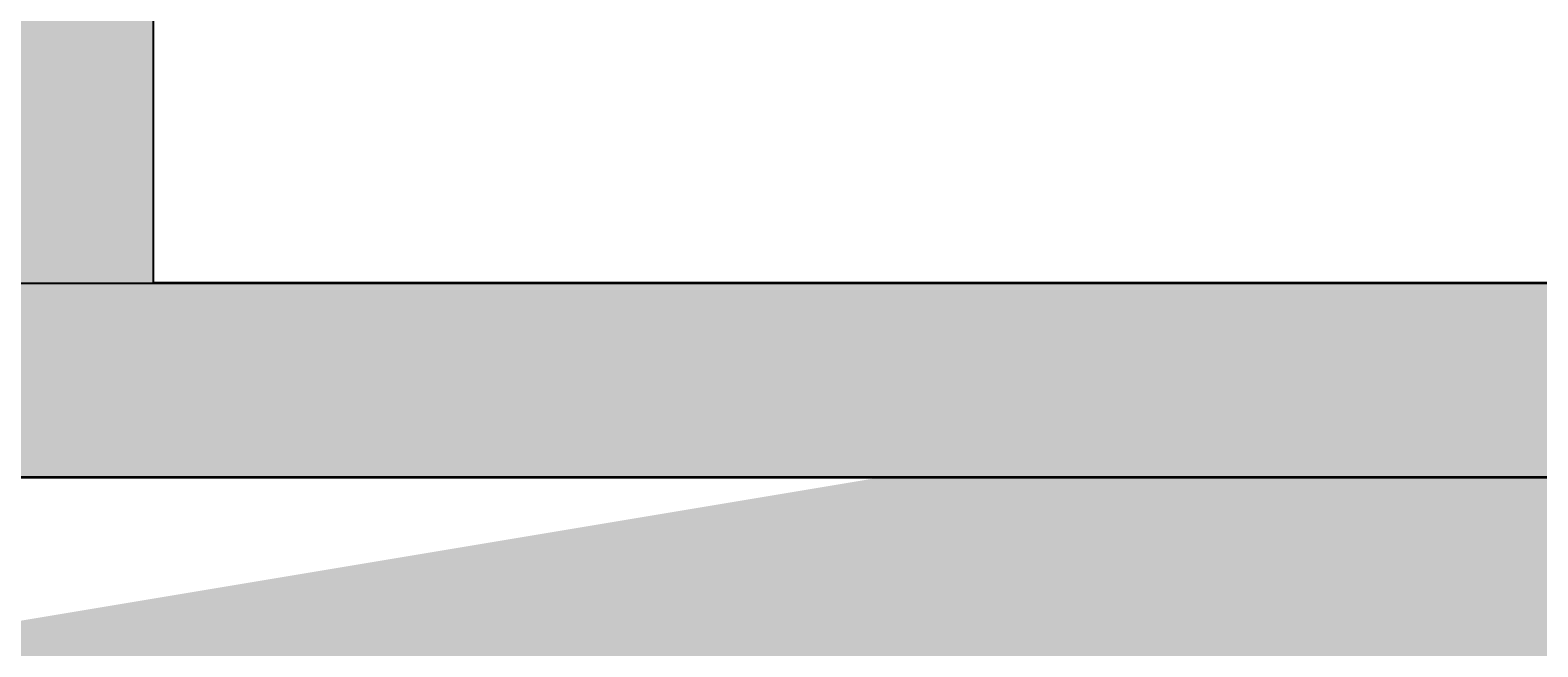
# Model space of a CAD drawing. Units: millimetres. Extents: x -22994 to 29398, y -19990 to 20176.
# Tile 51 of 135: x 198 to 247, y 5 to 25. Entities that reach past the tile are written whole.
import ezdxf

# ---------------------------------------------------------------- set-up
doc = ezdxf.new("R2010")
doc.units = ezdxf.units.MM
doc.header["$MEASUREMENT"] = 0
for name, color, linetype, lineweight in [('M-DIMS', 2, 'Continuous', 18), ('M-EQPM', 7, 'Continuous', 25), ('M-EQPM-PATT', 7, 'Continuous', 18), ('S-FNDN', 7, 'Continuous', 35)]:
    doc.layers.add(name, color=color, linetype=linetype, lineweight=lineweight)
doc.styles.get("Standard").update_dxf_attribs({"font": 'arial.ttf'})
doc.dimstyles.get("Standard").update_dxf_attribs({"dimtxt": 0.18, "dimasz": 10000, "dimexe": 0.18, "dimexo": 0.0625, "dimgap": 0.09, "dimtad": 0, "dimtih": 1, "dimtoh": 1, "dimdec": 0, "dimzin": 0, "dimdsep": 46, "dimtxsty": 'Standard', "dimcen": 0.09, "dimadec": 0, "dimazin": 0, "dimtfac": 1, "dimtdec": 0, "dimtofl": 0, "dimtmove": 0, "dimatfit": 3, "dimfxl": 1, "dimtolj": 1, "dimtzin": 0, "dimlwd": 30, "dimarcsym": 0})

# ---------------------------------------------------------------- blocks, each defined once
blk = doc.blocks.new('*D2')
at = {"layer": 'Defpoints', "color": 0, "transparency": 16777216}
for p in [(6.677, 10.271), (290.852, 10.271), (290.852, -5.079)]:
    blk.add_point(p, dxfattribs=at)
at = {"layer": 'M-DIMS', "color": 0, "lineweight": -2, "transparency": 16777216}
for p, q in [((6.677, 10.209), (6.677, -5.259)), ((290.852, 10.209), (290.852, -5.259))]:
    blk.add_line(p, q, dxfattribs=at)
at = {"layer": 'M-DIMS', "color": 0, "lineweight": 30, "transparency": 16777216}
for p, q in [((-9993.323, -5.079), (-19993.323, -5.079)), ((10290.852, -5.079), (20290.852, -5.079))]:
    blk.add_line(p, q, dxfattribs=at)
at = {"layer": 'M-DIMS', "color": 0, "transparency": 16777216}
for points in [[(-9993.323, 1661.588), (-9993.323, -1671.745), (6.677, -5.079)], [(10290.852, 1661.588), (10290.852, -1671.745), (290.852, -5.079)]]:
    blk.add_solid(points, dxfattribs=at)
at = {"layer": 'M-DIMS', "color": 0, "transparency": 16777216, "insert": (148.765, -5.079), "char_height": 0.18, "attachment_point": 5}
blk.add_mtext('\\A1;284.2', dxfattribs=at)
blk = doc.blocks.new('*D3')
at = {"layer": 'Defpoints', "color": 0, "transparency": 16777216}
for p in [(110.265, 204.165), (110.265, 176.366), (95.833, 127.967)]:
    blk.add_point(p, dxfattribs=at)
at = {"layer": 'M-DIMS', "color": 0, "lineweight": -2, "transparency": 16777216}
for p, q in [((95.833, 128.03), (95.833, 204.345)), ((110.265, 176.429), (110.265, 204.345))]:
    blk.add_line(p, q, dxfattribs=at)
at = {"layer": 'M-DIMS', "color": 0, "lineweight": 30, "transparency": 16777216}
for p, q in [((-9904.167, 204.165), (-19904.167, 204.165)), ((10110.265, 204.165), (20110.265, 204.165))]:
    blk.add_line(p, q, dxfattribs=at)
at = {"layer": 'M-DIMS', "color": 0, "transparency": 16777216}
for points in [[(-9904.167, 1870.832), (-9904.167, -1462.501), (95.833, 204.165)], [(10110.265, 1870.832), (10110.265, -1462.501), (110.265, 204.165)]]:
    blk.add_solid(points, dxfattribs=at)
at = {"layer": 'M-DIMS', "color": 0, "transparency": 16777216, "insert": (103.049, 204.165), "char_height": 0.18, "attachment_point": 5}
blk.add_mtext('\\A1;14.432', dxfattribs=at)
blk = doc.blocks.new('*D4')
at = {"layer": 'Defpoints', "color": 0, "transparency": 16777216}
for p in [(116.265, 204.165), (110.265, 176.366), (116.265, 176.366)]:
    blk.add_point(p, dxfattribs=at)
at = {"layer": 'M-DIMS', "color": 0, "lineweight": -2, "transparency": 16777216}
for p, q in [((110.265, 176.429), (110.265, 204.345)), ((116.265, 176.429), (116.265, 204.345))]:
    blk.add_line(p, q, dxfattribs=at)
at = {"layer": 'M-DIMS', "color": 0, "lineweight": 30, "transparency": 16777216}
for p, q in [((-9889.735, 204.165), (-19889.735, 204.165)), ((10116.265, 204.165), (20116.265, 204.165))]:
    blk.add_line(p, q, dxfattribs=at)
at = {"layer": 'M-DIMS', "color": 0, "transparency": 16777216}
for points in [[(-9889.735, 1870.832), (-9889.735, -1462.501), (110.265, 204.165)], [(10116.265, 1870.832), (10116.265, -1462.501), (116.265, 204.165)]]:
    blk.add_solid(points, dxfattribs=at)
at = {"layer": 'M-DIMS', "color": 0, "transparency": 16777216, "insert": (113.265, 204.165), "char_height": 0.18, "attachment_point": 5}
blk.add_mtext('\\A1;6', dxfattribs=at)
blk = doc.blocks.new('*D5')
at = {"layer": 'Defpoints', "color": 0, "transparency": 16777216}
for p in [(181.265, 204.165), (116.265, 176.366), (181.265, 176.366)]:
    blk.add_point(p, dxfattribs=at)
at = {"layer": 'M-DIMS', "color": 0, "lineweight": -2, "transparency": 16777216}
for p, q in [((116.265, 176.429), (116.265, 204.345)), ((181.265, 176.429), (181.265, 204.345))]:
    blk.add_line(p, q, dxfattribs=at)
at = {"layer": 'M-DIMS', "color": 0, "lineweight": 30, "transparency": 16777216}
for p, q in [((-9883.735, 204.165), (-19883.735, 204.165)), ((10181.265, 204.165), (20181.265, 204.165))]:
    blk.add_line(p, q, dxfattribs=at)
at = {"layer": 'M-DIMS', "color": 0, "transparency": 16777216}
for points in [[(-9883.735, 1870.832), (-9883.735, -1462.501), (116.265, 204.165)], [(10181.265, 1870.832), (10181.265, -1462.501), (181.265, 204.165)]]:
    blk.add_solid(points, dxfattribs=at)
at = {"layer": 'M-DIMS', "color": 0, "transparency": 16777216, "insert": (148.765, 204.165), "char_height": 0.18, "attachment_point": 5}
blk.add_mtext('\\A1;65', dxfattribs=at)
blk = doc.blocks.new('*D6')
at = {"layer": 'Defpoints', "color": 0, "transparency": 16777216}
for p in [(187.265, 204.165), (181.265, 176.366), (187.265, 176.366)]:
    blk.add_point(p, dxfattribs=at)
at = {"layer": 'M-DIMS', "color": 0, "lineweight": -2, "transparency": 16777216}
for p, q in [((181.265, 176.429), (181.265, 204.345)), ((187.265, 176.429), (187.265, 204.345))]:
    blk.add_line(p, q, dxfattribs=at)
at = {"layer": 'M-DIMS', "color": 0, "lineweight": 30, "transparency": 16777216}
for p, q in [((-9818.735, 204.165), (-19818.735, 204.165)), ((10187.265, 204.165), (20187.265, 204.165))]:
    blk.add_line(p, q, dxfattribs=at)
at = {"layer": 'M-DIMS', "color": 0, "transparency": 16777216}
for points in [[(-9818.735, 1870.832), (-9818.735, -1462.501), (181.265, 204.165)], [(10187.265, 1870.832), (10187.265, -1462.501), (187.265, 204.165)]]:
    blk.add_solid(points, dxfattribs=at)
at = {"layer": 'M-DIMS', "color": 0, "transparency": 16777216, "insert": (184.265, 204.165), "char_height": 0.18, "attachment_point": 5}
blk.add_mtext('\\A1;6', dxfattribs=at)
blk = doc.blocks.new('*D7')
at = {"layer": 'Defpoints', "color": 0, "transparency": 16777216}
for p in [(201.697, 204.165), (187.265, 176.366), (201.697, 127.967)]:
    blk.add_point(p, dxfattribs=at)
at = {"layer": 'M-DIMS', "color": 0, "lineweight": -2, "transparency": 16777216}
for p, q in [((187.265, 176.429), (187.265, 204.345)), ((201.697, 128.03), (201.697, 204.345))]:
    blk.add_line(p, q, dxfattribs=at)
at = {"layer": 'M-DIMS', "color": 0, "lineweight": 30, "transparency": 16777216}
for p, q in [((-9812.735, 204.165), (-19812.735, 204.165)), ((10201.697, 204.165), (20201.697, 204.165))]:
    blk.add_line(p, q, dxfattribs=at)
at = {"layer": 'M-DIMS', "color": 0, "transparency": 16777216}
for points in [[(-9812.735, 1870.832), (-9812.735, -1462.501), (187.265, 204.165)], [(10201.697, 1870.832), (10201.697, -1462.501), (201.697, 204.165)]]:
    blk.add_solid(points, dxfattribs=at)
at = {"layer": 'M-DIMS', "color": 0, "transparency": 16777216, "insert": (194.481, 204.165), "char_height": 0.18, "attachment_point": 5}
blk.add_mtext('\\A1;14.432', dxfattribs=at)
blk = doc.blocks.new('*D8')
at = {"layer": 'Defpoints', "color": 0, "transparency": 16777216}
for p in [(227.648, 204.165), (227.648, 146.73), (201.697, 127.967)]:
    blk.add_point(p, dxfattribs=at)
at = {"layer": 'M-DIMS', "color": 0, "lineweight": -2, "transparency": 16777216}
for p, q in [((201.697, 128.03), (201.697, 204.345)), ((227.648, 146.792), (227.648, 204.345))]:
    blk.add_line(p, q, dxfattribs=at)
at = {"layer": 'M-DIMS', "color": 0, "lineweight": 30, "transparency": 16777216}
for p, q in [((-9798.303, 204.165), (-19798.303, 204.165)), ((10227.648, 204.165), (20227.648, 204.165))]:
    blk.add_line(p, q, dxfattribs=at)
at = {"layer": 'M-DIMS', "color": 0, "transparency": 16777216}
for points in [[(-9798.303, 1870.832), (-9798.303, -1462.501), (201.697, 204.165)], [(10227.648, 1870.832), (10227.648, -1462.501), (227.648, 204.165)]]:
    blk.add_solid(points, dxfattribs=at)
at = {"layer": 'M-DIMS', "color": 0, "transparency": 16777216, "insert": (214.673, 204.165), "char_height": 0.18, "attachment_point": 5}
blk.add_mtext('\\A1;25.95', dxfattribs=at)
blk = doc.blocks.new('*D9')
at = {"layer": 'Defpoints', "color": 0, "transparency": 16777216}
for p in [(187.265, 176.366), (306.202, 176.366), (290.852, 10.271)]:
    blk.add_point(p, dxfattribs=at)
at = {"layer": 'M-DIMS', "color": 0, "lineweight": 30, "transparency": 16777216}
for p, q in [((306.202, 10176.366), (306.202, 20176.366)), ((306.202, -9989.729), (306.202, -19989.729))]:
    blk.add_line(p, q, dxfattribs=at)
at = {"layer": 'M-DIMS', "color": 0, "lineweight": -2, "transparency": 16777216}
for p, q in [((187.327, 176.366), (306.382, 176.366)), ((290.915, 10.271), (306.382, 10.271))]:
    blk.add_line(p, q, dxfattribs=at)
at = {"layer": 'M-DIMS', "color": 0, "transparency": 16777216}
for points in [[(-1360.465, 10176.366), (1972.869, 10176.366), (306.202, 176.366)], [(-1360.465, -9989.729), (1972.869, -9989.729), (306.202, 10.271)]]:
    blk.add_solid(points, dxfattribs=at)
at = {"layer": 'M-DIMS', "color": 0, "transparency": 16777216, "insert": (306.202, 93.319), "char_height": 0.18, "attachment_point": 5}
blk.add_mtext('\\A1;166.1', dxfattribs=at)
blk = doc.blocks.new('*D10')
at = {"layer": 'Defpoints', "color": 0, "transparency": 16777216}
for p in [(125.65, 136.071), (133.346, 136.071), (133.346, -5.079)]:
    blk.add_point(p, dxfattribs=at)
at = {"layer": 'M-DIMS', "color": 0, "lineweight": -2, "transparency": 16777216}
for p, q in [((125.65, 136.009), (125.65, -5.259)), ((133.346, 136.009), (133.346, -5.259))]:
    blk.add_line(p, q, dxfattribs=at)
at = {"layer": 'M-DIMS', "color": 0, "lineweight": 30, "transparency": 16777216}
for p, q in [((-9874.35, -5.079), (-19874.35, -5.079)), ((10133.346, -5.079), (20133.346, -5.079))]:
    blk.add_line(p, q, dxfattribs=at)
at = {"layer": 'M-DIMS', "color": 0, "transparency": 16777216}
for points in [[(-9874.35, 1661.588), (-9874.35, -1671.745), (125.65, -5.079)], [(10133.346, 1661.588), (10133.346, -1671.745), (133.346, -5.079)]]:
    blk.add_solid(points, dxfattribs=at)
at = {"layer": 'M-DIMS', "color": 0, "transparency": 16777216, "insert": (129.498, -5.079), "char_height": 0.18, "attachment_point": 5}
blk.add_mtext('\\A1;7.696', dxfattribs=at)
blk = doc.blocks.new('*D11')
at = {"layer": 'Defpoints', "color": 0, "transparency": 16777216}
for p in [(133.346, 136.071), (135.65, 136.071), (135.65, -5.079)]:
    blk.add_point(p, dxfattribs=at)
at = {"layer": 'M-DIMS', "color": 0, "lineweight": -2, "transparency": 16777216}
for p, q in [((133.346, 136.009), (133.346, -5.259)), ((135.65, 136.009), (135.65, -5.259))]:
    blk.add_line(p, q, dxfattribs=at)
at = {"layer": 'M-DIMS', "color": 0, "lineweight": 30, "transparency": 16777216}
for p, q in [((-9866.654, -5.079), (-19866.654, -5.079)), ((10135.65, -5.079), (20135.65, -5.079))]:
    blk.add_line(p, q, dxfattribs=at)
at = {"layer": 'M-DIMS', "color": 0, "transparency": 16777216}
for points in [[(-9866.654, 1661.588), (-9866.654, -1671.745), (133.346, -5.079)], [(10135.65, 1661.588), (10135.65, -1671.745), (135.65, -5.079)]]:
    blk.add_solid(points, dxfattribs=at)
at = {"layer": 'M-DIMS', "color": 0, "transparency": 16777216, "insert": (134.498, -5.079), "char_height": 0.18, "attachment_point": 5}
blk.add_mtext('\\A1;2.304', dxfattribs=at)
blk = doc.blocks.new('*D12')
at = {"layer": 'Defpoints', "color": 0, "transparency": 16777216}
for p in [(135.65, 136.071), (145.65, 136.071), (145.65, -5.079)]:
    blk.add_point(p, dxfattribs=at)
at = {"layer": 'M-DIMS', "color": 0, "lineweight": -2, "transparency": 16777216}
for p, q in [((135.65, 136.009), (135.65, -5.259)), ((145.65, 136.009), (145.65, -5.259))]:
    blk.add_line(p, q, dxfattribs=at)
at = {"layer": 'M-DIMS', "color": 0, "lineweight": 30, "transparency": 16777216}
for p, q in [((-9864.35, -5.079), (-19864.35, -5.079)), ((10145.65, -5.079), (20145.65, -5.079))]:
    blk.add_line(p, q, dxfattribs=at)
at = {"layer": 'M-DIMS', "color": 0, "transparency": 16777216}
for points in [[(-9864.35, 1661.588), (-9864.35, -1671.745), (135.65, -5.079)], [(10145.65, 1661.588), (10145.65, -1671.745), (145.65, -5.079)]]:
    blk.add_solid(points, dxfattribs=at)
at = {"layer": 'M-DIMS', "color": 0, "transparency": 16777216, "insert": (140.65, -5.079), "char_height": 0.18, "attachment_point": 5}
blk.add_mtext('\\A1;10', dxfattribs=at)
blk = doc.blocks.new('*D13')
at = {"layer": 'Defpoints', "color": 0, "transparency": 16777216}
for p in [(145.65, 136.071), (155.65, 136.071), (155.65, -5.079)]:
    blk.add_point(p, dxfattribs=at)
at = {"layer": 'M-DIMS', "color": 0, "lineweight": -2, "transparency": 16777216}
for p, q in [((145.65, 136.009), (145.65, -5.259)), ((155.65, 136.009), (155.65, -5.259))]:
    blk.add_line(p, q, dxfattribs=at)
at = {"layer": 'M-DIMS', "color": 0, "lineweight": 30, "transparency": 16777216}
for p, q in [((-9854.35, -5.079), (-19854.35, -5.079)), ((10155.65, -5.079), (20155.65, -5.079))]:
    blk.add_line(p, q, dxfattribs=at)
at = {"layer": 'M-DIMS', "color": 0, "transparency": 16777216}
for points in [[(-9854.35, 1661.588), (-9854.35, -1671.745), (145.65, -5.079)], [(10155.65, 1661.588), (10155.65, -1671.745), (155.65, -5.079)]]:
    blk.add_solid(points, dxfattribs=at)
at = {"layer": 'M-DIMS', "color": 0, "transparency": 16777216, "insert": (150.65, -5.079), "char_height": 0.18, "attachment_point": 5}
blk.add_mtext('\\A1;10', dxfattribs=at)
blk = doc.blocks.new('*D14')
at = {"layer": 'Defpoints', "color": 0, "transparency": 16777216}
for p in [(155.65, 136.071), (165.65, 136.071), (165.65, -5.079)]:
    blk.add_point(p, dxfattribs=at)
at = {"layer": 'M-DIMS', "color": 0, "lineweight": -2, "transparency": 16777216}
for p, q in [((155.65, 136.009), (155.65, -5.259)), ((165.65, 136.009), (165.65, -5.259))]:
    blk.add_line(p, q, dxfattribs=at)
at = {"layer": 'M-DIMS', "color": 0, "lineweight": 30, "transparency": 16777216}
for p, q in [((-9844.35, -5.079), (-19844.35, -5.079)), ((10165.65, -5.079), (20165.65, -5.079))]:
    blk.add_line(p, q, dxfattribs=at)
at = {"layer": 'M-DIMS', "color": 0, "transparency": 16777216}
for points in [[(-9844.35, 1661.588), (-9844.35, -1671.745), (155.65, -5.079)], [(10165.65, 1661.588), (10165.65, -1671.745), (165.65, -5.079)]]:
    blk.add_solid(points, dxfattribs=at)
at = {"layer": 'M-DIMS', "color": 0, "transparency": 16777216, "insert": (160.65, -5.079), "char_height": 0.18, "attachment_point": 5}
blk.add_mtext('\\A1;10', dxfattribs=at)
blk = doc.blocks.new('*D15')
at = {"layer": 'Defpoints', "color": 0, "transparency": 16777216}
for p in [(173.346, 154.788), (173.346, 136.071), (306.202, 136.071)]:
    blk.add_point(p, dxfattribs=at)
at = {"layer": 'M-DIMS', "color": 0, "lineweight": 30, "transparency": 16777216}
for p, q in [((306.202, 10154.788), (306.202, 20154.788)), ((306.202, -9863.929), (306.202, -19863.929))]:
    blk.add_line(p, q, dxfattribs=at)
at = {"layer": 'M-DIMS', "color": 0, "lineweight": -2, "transparency": 16777216}
for p, q in [((173.408, 154.788), (306.382, 154.788)), ((173.408, 136.071), (306.382, 136.071))]:
    blk.add_line(p, q, dxfattribs=at)
at = {"layer": 'M-DIMS', "color": 0, "transparency": 16777216}
for points in [[(-1360.465, 10154.788), (1972.869, 10154.788), (306.202, 154.788)], [(-1360.465, -9863.929), (1972.869, -9863.929), (306.202, 136.071)]]:
    blk.add_solid(points, dxfattribs=at)
at = {"layer": 'M-DIMS', "color": 0, "transparency": 16777216, "insert": (306.202, 145.43), "char_height": 0.18, "attachment_point": 5}
blk.add_mtext('\\A1;18.717', dxfattribs=at)
blk = doc.blocks.new('*D16')
at = {"layer": 'Defpoints', "color": 0, "transparency": 16777216}
for p in [(120.17, 204.165), (110.466, 48.035), (120.17, 48.035)]:
    blk.add_point(p, dxfattribs=at)
at = {"layer": 'M-DIMS', "color": 0, "lineweight": -2, "transparency": 16777216}
for p, q in [((110.466, 48.097), (110.466, 204.345)), ((120.17, 48.097), (120.17, 204.345))]:
    blk.add_line(p, q, dxfattribs=at)
at = {"layer": 'M-DIMS', "color": 0, "lineweight": 30, "transparency": 16777216}
for p, q in [((-9889.534, 204.165), (-19889.534, 204.165)), ((10120.17, 204.165), (20120.17, 204.165))]:
    blk.add_line(p, q, dxfattribs=at)
at = {"layer": 'M-DIMS', "color": 0, "transparency": 16777216}
for points in [[(-9889.534, 1870.832), (-9889.534, -1462.501), (110.466, 204.165)], [(10120.17, 1870.832), (10120.17, -1462.501), (120.17, 204.165)]]:
    blk.add_solid(points, dxfattribs=at)
at = {"layer": 'M-DIMS', "color": 0, "transparency": 16777216, "insert": (115.318, 204.165), "char_height": 0.18, "attachment_point": 5}
blk.add_mtext('\\A1;9.704', dxfattribs=at)
blk = doc.blocks.new('*D17')
at = {"layer": 'Defpoints', "color": 0, "transparency": 16777216}
for p in [(126.17, 204.165), (120.17, 48.035), (126.17, 48.035)]:
    blk.add_point(p, dxfattribs=at)
at = {"layer": 'M-DIMS', "color": 0, "lineweight": -2, "transparency": 16777216}
for p, q in [((120.17, 48.097), (120.17, 204.345)), ((126.17, 48.097), (126.17, 204.345))]:
    blk.add_line(p, q, dxfattribs=at)
at = {"layer": 'M-DIMS', "color": 0, "lineweight": 30, "transparency": 16777216}
for p, q in [((-9879.83, 204.165), (-19879.83, 204.165)), ((10126.17, 204.165), (20126.17, 204.165))]:
    blk.add_line(p, q, dxfattribs=at)
at = {"layer": 'M-DIMS', "color": 0, "transparency": 16777216}
for points in [[(-9879.83, 1870.832), (-9879.83, -1462.501), (120.17, 204.165)], [(10126.17, 1870.832), (10126.17, -1462.501), (126.17, 204.165)]]:
    blk.add_solid(points, dxfattribs=at)
at = {"layer": 'M-DIMS', "color": 0, "transparency": 16777216, "insert": (123.17, 204.165), "char_height": 0.18, "attachment_point": 5}
blk.add_mtext('\\A1;6', dxfattribs=at)
blk = doc.blocks.new('*D18')
at = {"layer": 'Defpoints', "color": 0, "transparency": 16777216}
for p in [(132.17, 204.165), (126.17, 48.035), (132.17, 48.035)]:
    blk.add_point(p, dxfattribs=at)
at = {"layer": 'M-DIMS', "color": 0, "lineweight": -2, "transparency": 16777216}
for p, q in [((126.17, 48.097), (126.17, 204.345)), ((132.17, 48.097), (132.17, 204.345))]:
    blk.add_line(p, q, dxfattribs=at)
at = {"layer": 'M-DIMS', "color": 0, "lineweight": 30, "transparency": 16777216}
for p, q in [((-9873.83, 204.165), (-19873.83, 204.165)), ((10132.17, 204.165), (20132.17, 204.165))]:
    blk.add_line(p, q, dxfattribs=at)
at = {"layer": 'M-DIMS', "color": 0, "transparency": 16777216}
for points in [[(-9873.83, 1870.832), (-9873.83, -1462.501), (126.17, 204.165)], [(10132.17, 1870.832), (10132.17, -1462.501), (132.17, 204.165)]]:
    blk.add_solid(points, dxfattribs=at)
at = {"layer": 'M-DIMS', "color": 0, "transparency": 16777216, "insert": (129.17, 204.165), "char_height": 0.18, "attachment_point": 5}
blk.add_mtext('\\A1;6', dxfattribs=at)
blk = doc.blocks.new('*D19')
at = {"layer": 'Defpoints', "color": 0, "transparency": 16777216}
for p in [(138.17, 204.165), (132.17, 48.035), (138.17, 48.035)]:
    blk.add_point(p, dxfattribs=at)
at = {"layer": 'M-DIMS', "color": 0, "lineweight": -2, "transparency": 16777216}
for p, q in [((132.17, 48.097), (132.17, 204.345)), ((138.17, 48.097), (138.17, 204.345))]:
    blk.add_line(p, q, dxfattribs=at)
at = {"layer": 'M-DIMS', "color": 0, "lineweight": 30, "transparency": 16777216}
for p, q in [((-9867.83, 204.165), (-19867.83, 204.165)), ((10138.17, 204.165), (20138.17, 204.165))]:
    blk.add_line(p, q, dxfattribs=at)
at = {"layer": 'M-DIMS', "color": 0, "transparency": 16777216}
for points in [[(-9867.83, 1870.832), (-9867.83, -1462.501), (132.17, 204.165)], [(10138.17, 1870.832), (10138.17, -1462.501), (138.17, 204.165)]]:
    blk.add_solid(points, dxfattribs=at)
at = {"layer": 'M-DIMS', "color": 0, "transparency": 16777216, "insert": (135.17, 204.165), "char_height": 0.18, "attachment_point": 5}
blk.add_mtext('\\A1;6', dxfattribs=at)
blk = doc.blocks.new('*D20')
at = {"layer": 'Defpoints', "color": 0, "transparency": 16777216}
for p in [(144.17, 204.165), (138.17, 48.035), (144.17, 48.035)]:
    blk.add_point(p, dxfattribs=at)
at = {"layer": 'M-DIMS', "color": 0, "lineweight": -2, "transparency": 16777216}
for p, q in [((138.17, 48.097), (138.17, 204.345)), ((144.17, 48.097), (144.17, 204.345))]:
    blk.add_line(p, q, dxfattribs=at)
at = {"layer": 'M-DIMS', "color": 0, "lineweight": 30, "transparency": 16777216}
for p, q in [((-9861.83, 204.165), (-19861.83, 204.165)), ((10144.17, 204.165), (20144.17, 204.165))]:
    blk.add_line(p, q, dxfattribs=at)
at = {"layer": 'M-DIMS', "color": 0, "transparency": 16777216}
for points in [[(-9861.83, 1870.832), (-9861.83, -1462.501), (138.17, 204.165)], [(10144.17, 1870.832), (10144.17, -1462.501), (144.17, 204.165)]]:
    blk.add_solid(points, dxfattribs=at)
at = {"layer": 'M-DIMS', "color": 0, "transparency": 16777216, "insert": (141.17, 204.165), "char_height": 0.18, "attachment_point": 5}
blk.add_mtext('\\A1;6', dxfattribs=at)
blk = doc.blocks.new('*D21')
at = {"layer": 'Defpoints', "color": 0, "transparency": 16777216}
for p in [(149.116, 204.165), (144.17, 48.035), (149.116, 48.035)]:
    blk.add_point(p, dxfattribs=at)
at = {"layer": 'M-DIMS', "color": 0, "lineweight": -2, "transparency": 16777216}
for p, q in [((144.17, 48.097), (144.17, 204.345)), ((149.116, 48.097), (149.116, 204.345))]:
    blk.add_line(p, q, dxfattribs=at)
at = {"layer": 'M-DIMS', "color": 0, "lineweight": 30, "transparency": 16777216}
for p, q in [((-9855.83, 204.165), (-19855.83, 204.165)), ((10149.116, 204.165), (20149.116, 204.165))]:
    blk.add_line(p, q, dxfattribs=at)
at = {"layer": 'M-DIMS', "color": 0, "transparency": 16777216}
for points in [[(-9855.83, 1870.832), (-9855.83, -1462.501), (144.17, 204.165)], [(10149.116, 1870.832), (10149.116, -1462.501), (149.116, 204.165)]]:
    blk.add_solid(points, dxfattribs=at)
at = {"layer": 'M-DIMS', "color": 0, "transparency": 16777216, "insert": (146.643, 204.165), "char_height": 0.18, "attachment_point": 5}
blk.add_mtext('\\A1;4.945', dxfattribs=at)
blk = doc.blocks.new('*D22')
at = {"layer": 'Defpoints', "color": 0, "transparency": 16777216}
for p in [(149.116, 30.99), (155.116, 30.99), (155.116, -5.079)]:
    blk.add_point(p, dxfattribs=at)
at = {"layer": 'M-DIMS', "color": 0, "lineweight": -2, "transparency": 16777216}
for p, q in [((149.116, 30.927), (149.116, -5.259)), ((155.116, 30.927), (155.116, -5.259))]:
    blk.add_line(p, q, dxfattribs=at)
at = {"layer": 'M-DIMS', "color": 0, "lineweight": 30, "transparency": 16777216}
for p, q in [((-9850.884, -5.079), (-19850.884, -5.079)), ((10155.116, -5.079), (20155.116, -5.079))]:
    blk.add_line(p, q, dxfattribs=at)
at = {"layer": 'M-DIMS', "color": 0, "transparency": 16777216}
for points in [[(-9850.884, 1661.588), (-9850.884, -1671.745), (149.116, -5.079)], [(10155.116, 1661.588), (10155.116, -1671.745), (155.116, -5.079)]]:
    blk.add_solid(points, dxfattribs=at)
at = {"layer": 'M-DIMS', "color": 0, "transparency": 16777216, "insert": (152.116, -5.079), "char_height": 0.18, "attachment_point": 5}
blk.add_mtext('\\A1;6', dxfattribs=at)
blk = doc.blocks.new('*D23')
at = {"layer": 'Defpoints', "color": 0, "transparency": 16777216}
for p in [(155.116, 30.99), (161.116, 30.99), (161.116, -5.079)]:
    blk.add_point(p, dxfattribs=at)
at = {"layer": 'M-DIMS', "color": 0, "lineweight": -2, "transparency": 16777216}
for p, q in [((155.116, 30.927), (155.116, -5.259)), ((161.116, 30.927), (161.116, -5.259))]:
    blk.add_line(p, q, dxfattribs=at)
at = {"layer": 'M-DIMS', "color": 0, "lineweight": 30, "transparency": 16777216}
for p, q in [((-9844.884, -5.079), (-19844.884, -5.079)), ((10161.116, -5.079), (20161.116, -5.079))]:
    blk.add_line(p, q, dxfattribs=at)
at = {"layer": 'M-DIMS', "color": 0, "transparency": 16777216}
for points in [[(-9844.884, 1661.588), (-9844.884, -1671.745), (155.116, -5.079)], [(10161.116, 1661.588), (10161.116, -1671.745), (161.116, -5.079)]]:
    blk.add_solid(points, dxfattribs=at)
at = {"layer": 'M-DIMS', "color": 0, "transparency": 16777216, "insert": (158.116, -5.079), "char_height": 0.18, "attachment_point": 5}
blk.add_mtext('\\A1;6', dxfattribs=at)
blk = doc.blocks.new('*D24')
at = {"layer": 'Defpoints', "color": 0, "transparency": 16777216}
for p in [(161.116, 30.99), (166.439, 30.99), (166.439, -5.079)]:
    blk.add_point(p, dxfattribs=at)
at = {"layer": 'M-DIMS', "color": 0, "lineweight": -2, "transparency": 16777216}
for p, q in [((161.116, 30.927), (161.116, -5.259)), ((166.439, 30.927), (166.439, -5.259))]:
    blk.add_line(p, q, dxfattribs=at)
at = {"layer": 'M-DIMS', "color": 0, "lineweight": 30, "transparency": 16777216}
for p, q in [((-9838.884, -5.079), (-19838.884, -5.079)), ((10166.439, -5.079), (20166.439, -5.079))]:
    blk.add_line(p, q, dxfattribs=at)
at = {"layer": 'M-DIMS', "color": 0, "transparency": 16777216}
for points in [[(-9838.884, 1661.588), (-9838.884, -1671.745), (161.116, -5.079)], [(10166.439, 1661.588), (10166.439, -1671.745), (166.439, -5.079)]]:
    blk.add_solid(points, dxfattribs=at)
at = {"layer": 'M-DIMS', "color": 0, "transparency": 16777216, "insert": (163.777, -5.079), "char_height": 0.18, "attachment_point": 5}
blk.add_mtext('\\A1;5.323', dxfattribs=at)
blk = doc.blocks.new('*D25')
at = {"layer": 'Defpoints', "color": 0, "transparency": 16777216}
for p in [(166.439, 30.99), (172.439, 30.99), (172.439, -5.079)]:
    blk.add_point(p, dxfattribs=at)
at = {"layer": 'M-DIMS', "color": 0, "lineweight": -2, "transparency": 16777216}
for p, q in [((166.439, 30.927), (166.439, -5.259)), ((172.439, 30.927), (172.439, -5.259))]:
    blk.add_line(p, q, dxfattribs=at)
at = {"layer": 'M-DIMS', "color": 0, "lineweight": 30, "transparency": 16777216}
for p, q in [((-9833.561, -5.079), (-19833.561, -5.079)), ((10172.439, -5.079), (20172.439, -5.079))]:
    blk.add_line(p, q, dxfattribs=at)
at = {"layer": 'M-DIMS', "color": 0, "transparency": 16777216}
for points in [[(-9833.561, 1661.588), (-9833.561, -1671.745), (166.439, -5.079)], [(10172.439, 1661.588), (10172.439, -1671.745), (172.439, -5.079)]]:
    blk.add_solid(points, dxfattribs=at)
at = {"layer": 'M-DIMS', "color": 0, "transparency": 16777216, "insert": (169.439, -5.079), "char_height": 0.18, "attachment_point": 5}
blk.add_mtext('\\A1;6', dxfattribs=at)
blk = doc.blocks.new('*D26')
at = {"layer": 'Defpoints', "color": 0, "transparency": 16777216}
for p in [(172.439, 30.99), (178.439, 30.99), (178.439, -5.079)]:
    blk.add_point(p, dxfattribs=at)
at = {"layer": 'M-DIMS', "color": 0, "lineweight": -2, "transparency": 16777216}
for p, q in [((172.439, 30.927), (172.439, -5.259)), ((178.439, 30.927), (178.439, -5.259))]:
    blk.add_line(p, q, dxfattribs=at)
at = {"layer": 'M-DIMS', "color": 0, "lineweight": 30, "transparency": 16777216}
for p, q in [((-9827.561, -5.079), (-19827.561, -5.079)), ((10178.439, -5.079), (20178.439, -5.079))]:
    blk.add_line(p, q, dxfattribs=at)
at = {"layer": 'M-DIMS', "color": 0, "transparency": 16777216}
for points in [[(-9827.561, 1661.588), (-9827.561, -1671.745), (172.439, -5.079)], [(10178.439, 1661.588), (10178.439, -1671.745), (178.439, -5.079)]]:
    blk.add_solid(points, dxfattribs=at)
at = {"layer": 'M-DIMS', "color": 0, "transparency": 16777216, "insert": (175.439, -5.079), "char_height": 0.18, "attachment_point": 5}
blk.add_mtext('\\A1;6', dxfattribs=at)
blk = doc.blocks.new('*D27')
at = {"layer": 'Defpoints', "color": 0, "transparency": 16777216}
for p in [(178.439, 30.99), (188.117, 30.99), (188.117, -5.079)]:
    blk.add_point(p, dxfattribs=at)
at = {"layer": 'M-DIMS', "color": 0, "lineweight": -2, "transparency": 16777216}
for p, q in [((178.439, 30.927), (178.439, -5.259)), ((188.117, 30.927), (188.117, -5.259))]:
    blk.add_line(p, q, dxfattribs=at)
at = {"layer": 'M-DIMS', "color": 0, "lineweight": 30, "transparency": 16777216}
for p, q in [((-9821.561, -5.079), (-19821.561, -5.079)), ((10188.117, -5.079), (20188.117, -5.079))]:
    blk.add_line(p, q, dxfattribs=at)
at = {"layer": 'M-DIMS', "color": 0, "transparency": 16777216}
for points in [[(-9821.561, 1661.588), (-9821.561, -1671.745), (178.439, -5.079)], [(10188.117, 1661.588), (10188.117, -1671.745), (188.117, -5.079)]]:
    blk.add_solid(points, dxfattribs=at)
at = {"layer": 'M-DIMS', "color": 0, "transparency": 16777216, "insert": (183.278, -5.079), "char_height": 0.18, "attachment_point": 5}
blk.add_mtext('\\A1;9.679', dxfattribs=at)
blk = doc.blocks.new('*D28')
at = {"layer": 'Defpoints', "color": 0, "transparency": 16777216}
for p in [(188.117, 48.035), (306.202, 48.035), (188.117, 30.99)]:
    blk.add_point(p, dxfattribs=at)
at = {"layer": 'M-DIMS', "color": 0, "lineweight": 30, "transparency": 16777216}
for p, q in [((306.202, 10048.035), (306.202, 20048.035)), ((306.202, -9969.01), (306.202, -19969.01))]:
    blk.add_line(p, q, dxfattribs=at)
at = {"layer": 'M-DIMS', "color": 0, "lineweight": -2, "transparency": 16777216}
for p, q in [((188.18, 48.035), (306.382, 48.035)), ((188.18, 30.99), (306.382, 30.99))]:
    blk.add_line(p, q, dxfattribs=at)
at = {"layer": 'M-DIMS', "color": 0, "transparency": 16777216}
for points in [[(-1360.465, 10048.035), (1972.869, 10048.035), (306.202, 48.035)], [(-1360.465, -9969.01), (1972.869, -9969.01), (306.202, 30.99)]]:
    blk.add_solid(points, dxfattribs=at)
at = {"layer": 'M-DIMS', "color": 0, "transparency": 16777216, "insert": (306.202, 39.512), "char_height": 0.18, "attachment_point": 5}
blk.add_mtext('\\A1;17.045', dxfattribs=at)
blk = doc.blocks.new('*D29')
at = {"layer": 'Defpoints', "color": 0, "transparency": 16777216}
for p in [(36.801, 80.045), (64.03, 80.045)]:
    blk.add_point(p, dxfattribs=at)
at = {"layer": 'M-DIMS', "color": 0, "lineweight": -2, "transparency": 16777216}
for p, q in [((50.325, 80.045), (50.505, 80.045)), ((50.415, 79.955), (50.415, 80.135))]:
    blk.add_line(p, q, dxfattribs=at)
at = {"layer": 'M-DIMS', "color": 0, "lineweight": 30, "transparency": 16777216}
blk.add_line((20064.03, 80.03), (10064.03, 80.038), dxfattribs=at)
at = {"layer": 'M-DIMS', "color": 0, "transparency": 16777216}
blk.add_solid([(10064.031, 1746.704), (10064.028, -1586.629), (64.03, 80.045)], dxfattribs=at)
at = {"layer": 'M-DIMS', "color": 0, "transparency": 16777216, "insert": (20064.521, 80.03), "char_height": 0.18, "attachment_point": 5}
blk.add_mtext('\\A1;∅27.23', dxfattribs=at)
blk = doc.blocks.new('*D30')
at = {"layer": 'Defpoints', "color": 0, "transparency": 16777216}
for p in [(216.315, 146.729), (238.982, 146.73)]:
    blk.add_point(p, dxfattribs=at)
at = {"layer": 'M-DIMS', "color": 0, "lineweight": 30, "transparency": 16777216}
blk.add_line((20238.982, 147.496), (10238.982, 147.113), dxfattribs=at)
at = {"layer": 'M-DIMS', "color": 0, "lineweight": -2, "transparency": 16777216}
for p, q in [((227.558, 146.73), (227.738, 146.73)), ((227.648, 146.64), (227.648, 146.82))]:
    blk.add_line(p, q, dxfattribs=at)
at = {"layer": 'M-DIMS', "color": 0, "transparency": 16777216}
blk.add_solid([(10238.918, 1813.78), (10239.046, -1519.554), (238.982, 146.73)], dxfattribs=at)
at = {"layer": 'M-DIMS', "color": 0, "transparency": 16777216, "insert": (20239.544, 147.496), "char_height": 0.18, "attachment_point": 5}
blk.add_mtext('\\A1;∅22.667', dxfattribs=at)
blk = doc.blocks.new('*D31')
at = {"layer": 'Defpoints', "color": 0, "transparency": 16777216}
for p in [(223.164, 146.729), (232.133, 146.73)]:
    blk.add_point(p, dxfattribs=at)
at = {"layer": 'M-DIMS', "color": 0, "lineweight": 30, "transparency": 16777216}
blk.add_line((20232.133, 148.666), (10232.133, 147.698), dxfattribs=at)
at = {"layer": 'M-DIMS', "color": 0, "lineweight": -2, "transparency": 16777216}
for p, q in [((227.558, 146.73), (227.738, 146.73)), ((227.648, 146.64), (227.648, 146.82))]:
    blk.add_line(p, q, dxfattribs=at)
at = {"layer": 'M-DIMS', "color": 0, "transparency": 16777216}
blk.add_solid([(10231.971, 1814.364), (10232.294, -1518.969), (232.133, 146.73)], dxfattribs=at)
at = {"layer": 'M-DIMS', "color": 0, "transparency": 16777216, "insert": (20232.625, 148.666), "char_height": 0.18, "attachment_point": 5}
blk.add_mtext('\\A1;∅8.969', dxfattribs=at)
blk = doc.blocks.new('*D33')
at = {"layer": 'Defpoints', "color": 0, "transparency": 16777216}
for p in [(229.561, 154.377), (232.997, 153.351)]:
    blk.add_point(p, dxfattribs=at)
at = {"layer": 'M-DIMS', "color": 0, "lineweight": -2, "transparency": 16777216}
for p, q in [((229.471, 154.377), (229.651, 154.377)), ((229.561, 154.287), (229.561, 154.467))]:
    blk.add_line(p, q, dxfattribs=at)
at = {"layer": 'M-DIMS', "color": 0, "lineweight": 30, "transparency": 16777216}
for p, q in [((19396.339, -5570.838), (9814.668, -2708.743)), ((29396.339, -5570.838), (19396.339, -5570.838))]:
    blk.add_line(p, q, dxfattribs=at)
at = {"layer": 'M-DIMS', "color": 0, "transparency": 16777216}
blk.add_solid([(10291.684, -1111.798), (9337.652, -4305.689), (232.997, 153.351)], dxfattribs=at)
at = {"layer": 'M-DIMS', "color": 0, "transparency": 16777216, "insert": (29397.012, -5570.838), "char_height": 0.18, "attachment_point": 5}
blk.add_mtext('\\A1;6X R3.586', dxfattribs=at)
blk = doc.blocks.new('*D37')
at = {"layer": 'Defpoints', "color": 0, "transparency": 16777216}
for p in [(54.834, 118.615), (59.494, 118.614)]:
    blk.add_point(p, dxfattribs=at)
at = {"layer": 'M-DIMS', "color": 0, "lineweight": -2, "transparency": 16777216}
for p, q in [((57.074, 118.614), (57.254, 118.614)), ((57.164, 118.524), (57.164, 118.704))]:
    blk.add_line(p, q, dxfattribs=at)
at = {"layer": 'M-DIMS', "color": 0, "lineweight": 30, "transparency": 16777216}
blk.add_line((20059.493, 116.253), (10059.494, 117.434), dxfattribs=at)
at = {"layer": 'M-DIMS', "color": 0, "transparency": 16777216}
blk.add_solid([(10059.69, 1784.1), (10059.297, -1549.233), (59.494, 118.614)], dxfattribs=at)
at = {"layer": 'M-DIMS', "color": 0, "transparency": 16777216, "insert": (20059.985, 116.253), "char_height": 0.18, "attachment_point": 5}
blk.add_mtext('\\A1;∅4.659', dxfattribs=at)

msp = doc.modelspace()

# ---------------------------------------------------------------- hatches: boundary and pattern name
at = {"layer": 'M-EQPM-PATT'}
h = msp.add_hatch(color=256, dxfattribs=at)
h.set_gradient(color1=(205, 32, 39), color2=(205, 32, 39), tint=1)
h.paths.add_polyline_path([(116.2647, 150.3662), (116.2647, 170.3662), (116.2647, 176.3662), (110.2647, 176.3662), (110.2647, 152.0276), (95.8327, 127.967), (95.8327, 16.6063), (201.6967, 16.6063), (201.6967, 127.967), (187.2647, 152.0276), (187.2647, 176.3662), (181.2647, 176.3662), (181.2647, 170.3662), (181.2647, 150.3662), (195.6967, 126.3055), (195.6967, 22.6063), (101.8327, 22.6063), (101.8327, 126.3055)])
h.paths.add_polyline_path([(185.2208, 88.6347), (101.8327, 88.6347), (101.8327, 87.6347), (182.8066, 87.6347), (178.7313, 83.5594), (195.6967, 83.5594), (195.6967, 84.5594), (181.1455, 84.5594)], flags=17)
h.paths.add_polyline_path([(95.8327, 88.6347), (60.9779, 88.6347, -0.0228552), (61.7178, 87.6347), (95.8327, 87.6347)])
h.paths.add_polyline_path([(215.6212, 86.5189), (215.6212, 80.5999), (220.5095, 83.5594)])
h.paths.add_polyline_path([(215.6212, 84.5594), (201.6967, 84.5594), (201.6967, 83.5594), (215.6212, 83.5594)])
h.paths.add_polyline_path([(225.3978, 86.5189), (220.5095, 83.5594), (225.3978, 80.5999)])
h.paths.add_polyline_path([(231.6256, 84.5594), (225.3978, 84.5594), (225.3978, 83.5594), (231.6256, 83.5594)])
at = {"layer": 'S-FNDN'}
h = msp.add_hatch(color=256, dxfattribs=at)
h.set_gradient(color1=(241, 235, 31), color2=(244, 238, 81), tint=1, name='CYLINDER')
h.paths.add_polyline_path([(290.852, 16.6063), (201.6967, 16.6063), (95.8327, 16.6063), (81.8485, 16.6063), (82.3691, 10.2713), (290.852, 10.2713)])
h.paths.add_polyline_path([(81.8485, 16.6063), (60.8206, 16.6063), (62.0909, 10.2713), (82.3691, 10.2713)])
h.paths.add_polyline_path([(60.8206, 16.6063), (6.6773, 16.6063), (6.6773, 10.2713), (62.0909, 10.2713)])

# ---------------------------------------------------------------- linework, layer by layer
at = {"layer": 'M-EQPM'}
msp.add_lwpolyline([(110.2647, 176.3662), (110.2647, 152.0276), (95.8327, 127.967), (95.8327, 16.6063), (201.6967, 16.6063), (201.6967, 127.967), (187.2647, 152.0276), (187.2647, 176.3662)], close=True, dxfattribs=at)
at = {"layer": 'S-FNDN'}
msp.add_lwpolyline([(95.8327, 16.6063), (6.6773, 16.6063), (6.6773, 10.2713), (290.852, 10.2713), (290.852, 16.6063), (201.6967, 16.6063)], dxfattribs=at)

# ---------------------------------------------------------------- dimensions: what is measured, and where the dimension line sits
at = {"layer": 'M-DIMS'}
for base, p1, p2, override, picture, middle in [((306.202, 176.3662), (290.852, 10.2713), (187.2647, 176.3662), {"dimdec": 1, "dimlfac": 1, "dimrnd": 0, "dimzin": 0, "dimdsep": 46, "dimlunit": 2}, '*D9', (306.202, 93.3187)), ((306.202, 136.0713), (173.3459, 154.788), (173.3459, 136.0713), {"dimdec": 3, "dimlfac": 1, "dimrnd": 0, "dimzin": 0, "dimdsep": 46, "dimlunit": 2}, '*D15', (306.202, 145.4297)), ((306.202, 48.0349), (188.1175, 30.9895), (188.1175, 48.0349), {"dimdec": 3, "dimlfac": 1, "dimrnd": 0, "dimzin": 0, "dimdsep": 46, "dimlunit": 2}, '*D28', (306.202, 39.5122))]:
    dim = msp.add_linear_dim(base=base, p1=p1, p2=p2, angle=90, dimstyle='Standard', override=override, dxfattribs=at)
    dim.commit()
    dim.dimension.update_dxf_attribs({"geometry": picture, "text_midpoint": middle})
for base, p1, p2, override, picture, middle in [((110.2647, 204.1654), (95.8327, 127.967), (110.2647, 176.3662), {"dimdec": 3, "dimlfac": 1, "dimrnd": 0, "dimzin": 0, "dimdsep": 46, "dimlunit": 2}, '*D3', (103.0487, 204.1654)), ((116.2647, 204.1654), (110.2647, 176.3662), (116.2647, 176.3662), {"dimdec": 0, "dimlfac": 1, "dimrnd": 0, "dimzin": 0, "dimdsep": 46, "dimlunit": 2}, '*D4', (113.2647, 204.1654)), ((120.1702, 204.1654), (110.4658, 48.0349), (120.1702, 48.0349), {"dimdec": 3, "dimlfac": 1, "dimrnd": 0, "dimzin": 0, "dimdsep": 46, "dimlunit": 2}, '*D16', (115.318, 204.1654)), ((181.2647, 204.1654), (116.2647, 176.3662), (181.2647, 176.3662), {"dimdec": 0, "dimlfac": 1, "dimrnd": 0, "dimzin": 0, "dimdsep": 46, "dimlunit": 2}, '*D5', (148.7647, 204.1654)), ((126.1702, 204.1654), (120.1702, 48.0349), (126.1702, 48.0349), {"dimdec": 0, "dimlfac": 1, "dimrnd": 0, "dimzin": 0, "dimdsep": 46, "dimlunit": 2}, '*D17', (123.1702, 204.1654)), ((132.1702, 204.1654), (126.1702, 48.0349), (132.1702, 48.0349), {"dimdec": 0, "dimlfac": 1, "dimrnd": 0, "dimzin": 0, "dimdsep": 46, "dimlunit": 2}, '*D18', (129.1702, 204.1654)), ((138.1702, 204.1654), (132.1702, 48.0349), (138.1702, 48.0349), {"dimdec": 0, "dimlfac": 1, "dimrnd": 0, "dimzin": 0, "dimdsep": 46, "dimlunit": 2}, '*D19', (135.1702, 204.1654)), ((144.1702, 204.1654), (138.1702, 48.0349), (144.1702, 48.0349), {"dimdec": 0, "dimlfac": 1, "dimrnd": 0, "dimzin": 0, "dimdsep": 46, "dimlunit": 2}, '*D20', (141.1702, 204.1654)), ((149.11567, 204.16539), (144.17023, 48.03494), (149.11567, 48.03494), {"dimdec": 3, "dimlfac": 1, "dimrnd": 0, "dimzin": 0, "dimdsep": 46, "dimlunit": 2}, '*D21', (146.64295, 204.16539)), ((187.2647, 204.1654), (181.2647, 176.3662), (187.2647, 176.3662), {"dimdec": 0, "dimlfac": 1, "dimrnd": 0, "dimzin": 0, "dimdsep": 46, "dimlunit": 2}, '*D6', (184.2647, 204.1654)), ((201.6967, 204.1654), (187.2647, 176.3662), (201.6967, 127.967), {"dimdec": 3, "dimlfac": 1, "dimrnd": 0, "dimzin": 0, "dimdsep": 46, "dimlunit": 2}, '*D7', (194.4807, 204.1654)), ((227.6485, 204.1654), (201.6967, 127.967), (227.6485, 146.7296), {"dimdec": 2, "dimlfac": 1, "dimrnd": 0, "dimzin": 0, "dimdsep": 46, "dimlunit": 2}, '*D8', (214.6726, 204.1654)), ((290.852, -5.0787), (6.6773, 10.2713), (290.852, 10.2713), {"dimdec": 1, "dimlfac": 1, "dimrnd": 0, "dimzin": 0, "dimdsep": 46, "dimlunit": 2}, '*D2', (148.7647, -5.0787)), ((133.3459, -5.0787), (125.6498, 136.0713), (133.3459, 136.0713), {"dimdec": 3, "dimlfac": 1, "dimrnd": 0, "dimzin": 0, "dimdsep": 46, "dimlunit": 2}, '*D10', (129.4978, -5.0787)), ((135.6498, -5.0787), (133.3459, 136.0713), (135.6498, 136.0713), {"dimdec": 3, "dimlfac": 1, "dimrnd": 0, "dimzin": 0, "dimdsep": 46, "dimlunit": 2}, '*D11', (134.4978, -5.0787)), ((145.6498, -5.0787), (135.6498, 136.0713), (145.6498, 136.0713), {"dimdec": 0, "dimlfac": 1, "dimrnd": 0, "dimzin": 0, "dimdsep": 46, "dimlunit": 2}, '*D12', (140.6498, -5.0787)), ((155.6498, -5.0787), (145.6498, 136.0713), (155.6498, 136.0713), {"dimdec": 0, "dimlfac": 1, "dimrnd": 0, "dimzin": 0, "dimdsep": 46, "dimlunit": 2}, '*D13', (150.6498, -5.0787)), ((155.1157, -5.0787), (149.1157, 30.9895), (155.1157, 30.9895), {"dimdec": 0, "dimlfac": 1, "dimrnd": 0, "dimzin": 0, "dimdsep": 46, "dimlunit": 2}, '*D22', (152.1157, -5.0787)), ((161.1157, -5.0787), (155.1157, 30.9895), (161.1157, 30.9895), {"dimdec": 0, "dimlfac": 1, "dimrnd": 0, "dimzin": 0, "dimdsep": 46, "dimlunit": 2}, '*D23', (158.1157, -5.0787)), ((165.6498, -5.0787), (155.6498, 136.0713), (165.6498, 136.0713), {"dimdec": 0, "dimlfac": 1, "dimrnd": 0, "dimzin": 0, "dimdsep": 46, "dimlunit": 2}, '*D14', (160.6498, -5.0787)), ((166.4387, -5.0787), (161.1157, 30.9895), (166.4387, 30.9895), {"dimdec": 3, "dimlfac": 1, "dimrnd": 0, "dimzin": 0, "dimdsep": 46, "dimlunit": 2}, '*D24', (163.7772, -5.0787)), ((172.4387, -5.0787), (166.4387, 30.9895), (172.4387, 30.9895), {"dimdec": 0, "dimlfac": 1, "dimrnd": 0, "dimzin": 0, "dimdsep": 46, "dimlunit": 2}, '*D25', (169.4387, -5.0787)), ((178.4387, -5.0787), (172.4387, 30.9895), (178.4387, 30.9895), {"dimdec": 0, "dimlfac": 1, "dimrnd": 0, "dimzin": 0, "dimdsep": 46, "dimlunit": 2}, '*D26', (175.4387, -5.0787)), ((188.1175, -5.0787), (178.4387, 30.9895), (188.1175, 30.9895), {"dimdec": 3, "dimlfac": 1, "dimrnd": 0, "dimzin": 0, "dimdsep": 46, "dimlunit": 2}, '*D27', (183.2781, -5.0787))]:
    dim = msp.add_linear_dim(base=base, p1=p1, p2=p2, dimstyle='Standard', override=override, dxfattribs=at)
    dim.commit()
    dim.dimension.update_dxf_attribs({"geometry": picture, "text_midpoint": middle})
for p1, p2, picture, middle in [((223.1641, 146.7291), (232.1328, 146.73), '*D31', (20232.1327, 148.6656)), ((216.3148, 146.7291), (238.9821, 146.73), '*D30', (20238.9821, 147.4959))]:
    dim = msp.add_diameter_dim_2p(p1=p1, p2=p2, dimstyle='Standard', override={"dimdec": 3, "dimlfac": 1, "dimrnd": 0, "dimzin": 0, "dimdsep": 46, "dimlunit": 2}, dxfattribs=at)
    dim.commit()
    dim.dimension.update_dxf_attribs({"geometry": picture, "text_midpoint": middle, "dimtype": 163})
for p1, p2, override, picture, middle in [((54.8343, 118.6145), (59.4936, 118.614), {"dimdec": 3, "dimlfac": 1, "dimrnd": 0, "dimzin": 0, "dimdsep": 46, "dimlunit": 2}, '*D37', (20059.4934, 116.2531)), ((36.8006, 80.045), (64.0296, 80.045), {"dimdec": 2, "dimlfac": 1, "dimrnd": 0, "dimzin": 0, "dimdsep": 46, "dimlunit": 2}, '*D29', (20064.0296, 80.0303))]:
    dim = msp.add_diameter_dim_2p(p1=p1, p2=p2, dimstyle='Standard', override=override, dxfattribs=at)
    dim.commit()
    dim.dimension.update_dxf_attribs({"geometry": picture, "text_midpoint": middle})
dim = msp.add_radius_dim(center=(229.5613, 154.3773), mpoint=(232.9972, 153.3509), text='6X <>', dimstyle='Standard', override={"dimdec": 3, "dimlfac": 1, "dimrnd": 0, "dimzin": 0, "dimdsep": 46, "dimlunit": 2}, dxfattribs=at)
dim.commit()
dim.dimension.update_dxf_attribs({"geometry": '*D33', "text_midpoint": (29397.0125, -5570.8378)})

doc.saveas('drawing.dxf')
